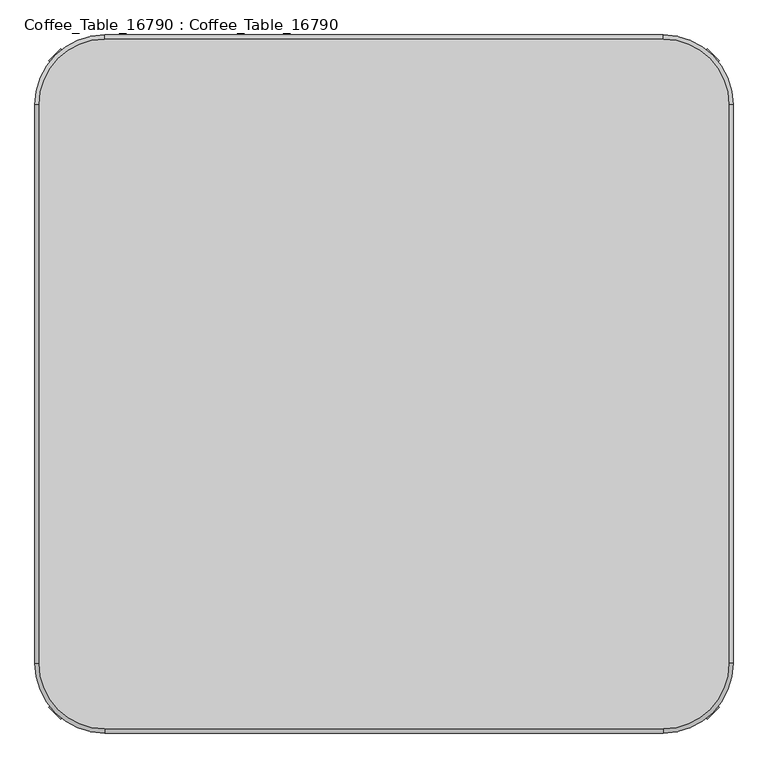
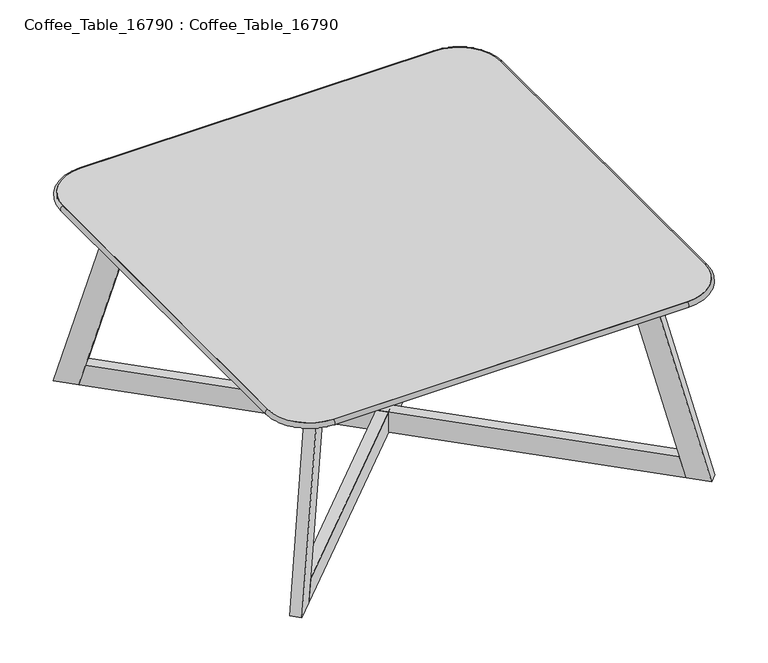
"""IFC4 building model written with IfcOpenShell, lengths in millimetres: furniture geometry, Coffee_Table_16790 : Coffee_Table_16790."""

from ifc_helpers import new_model, si_unit, point, frame, frame_2d, origin, place, context, project, spatial, polyline, circle_curve, ellipse_curve, trimmed, segment, composite_curve, outline, extrude, source, transform, mapped, element, save
from ifc_brep_helpers import plane_surface, cylinder_surface, revolved_surface, advanced_brep


def coffee_table_16790_coffee_table_16790_723536ea(model_context):
    return source(origin(), model_context, "Body", "SolidModel", [
        extrude(outline(composite_curve([segment(trimmed(circle_curve(frame_2d((400.0, 400.0)), 94.0), [point((400.0, 494.0))], [point((494.0, 400.0))], False, "CARTESIAN"), True, "CONTINUOUS"), segment(polyline([(494.0, 400.0), (494.0, -400.0)]), True, "CONTINUOUS"), segment(trimmed(circle_curve(frame_2d((400.0, -400.0)), 94.0), [point((494.0, -400.0))], [point((400.0, -494.0))], False, "CARTESIAN"), True, "CONTINUOUS"), segment(polyline([(400.0, -494.0), (-400.0, -494.0)]), True, "CONTINUOUS"), segment(trimmed(circle_curve(frame_2d((-400.0, -400.0)), 94.0), [point((-400.0, -494.0))], [point((-494.0, -400.0))], False, "CARTESIAN"), True, "CONTINUOUS"), segment(polyline([(-494.0, -400.0), (-494.0, 400.0)]), True, "CONTINUOUS"), segment(trimmed(circle_curve(frame_2d((-400.0, 400.0)), 94.0), [point((-494.0, 400.0))], [point((-400.0, 494.0))], False, "CARTESIAN"), True, "CONTINUOUS"), segment(polyline([(-400.0, 494.0), (400.0, 494.0)]), True, "CONTINUOUS")], self_intersect=False)), frame((0.0, 0.0, 448.0), z_axis=(0.0, 0.0, 1.0), x_axis=(1.0, 0.0, 0.0)), (0.0, 0.0, 1.0), 12.0),
        advanced_brep(
        [(-494.0, 400.0, 460.0), (-494.0, 400.0, 448.0), (-494.0, -400.0, 448.0), (-494.0, -400.0, 460.0), (-400.0, -494.0, 460.0), (-400.0, -494.0, 448.0), (400.0, -494.0, 448.0), (400.0, -494.0, 460.0), (494.0, -400.0, 460.0), (494.0, -400.0, 448.0), (494.0, 400.0, 448.0), (494.0, 400.0, 460.0), (400.0, 494.0, 460.0), (400.0, 494.0, 448.0), (-400.0, 494.0, 448.0), (-400.0, 494.0, 460.0)],
        [
            (0, 1, circle_curve(frame((-494.0, 400.0, 454.0), z_axis=(0.0, -1.0, 0.0), x_axis=(1.0, 0.0, 0.0)), 6.0)),
            (1, 2),
            (2, 3, circle_curve(frame((-494.0, -400.0, 454.0), z_axis=(0.0, 1.0, 0.0), x_axis=(1.0, 0.0, 0.0)), 6.0)),
            (3, 0),
            (1, 0),
            (3, 2),
            (4, 3, circle_curve(frame((-400.0, -400.0, 460.0), z_axis=(0.0, 0.0, -1.0), x_axis=(-1.0, 0.0, 0.0)), 94.0)),
            (2, 5, circle_curve(frame((-400.0, -400.0, 448.0), z_axis=(0.0, 0.0, 1.0), x_axis=(-1.0, 0.0, 0.0)), 94.0)),
            (5, 4, circle_curve(frame((-400.0, -494.0, 454.0), z_axis=(-1.0, 0.0, 0.0), x_axis=(0.0, 1.0, 0.0)), 6.0)),
            (4, 5),
            (5, 6),
            (6, 7, circle_curve(frame((400.0, -494.0, 454.0), z_axis=(-1.0, 0.0, 0.0), x_axis=(0.0, 1.0, 0.0)), 6.0)),
            (7, 4),
            (7, 6),
            (8, 7, circle_curve(frame((400.0, -400.0, 460.0), z_axis=(0.0, 0.0, -1.0), x_axis=(0.0, -1.0, 0.0)), 94.0)),
            (6, 9, circle_curve(frame((400.0, -400.0, 448.0), z_axis=(0.0, 0.0, 1.0), x_axis=(0.0, -1.0, 0.0)), 94.0)),
            (9, 8, circle_curve(frame((494.0, -400.0, 454.0), z_axis=(0.0, -1.0, 0.0), x_axis=(-1.0, 0.0, 0.0)), 6.0)),
            (8, 9),
            (9, 10),
            (10, 11, circle_curve(frame((494.0, 400.0, 454.0), z_axis=(0.0, -1.0, 0.0), x_axis=(-1.0, 0.0, 0.0)), 6.0)),
            (11, 8),
            (11, 10),
            (12, 11, circle_curve(frame((400.0, 400.0, 460.0), z_axis=(0.0, 0.0, -1.0), x_axis=(1.0, 0.0, 0.0)), 94.0)),
            (10, 13, circle_curve(frame((400.0, 400.0, 448.0), z_axis=(0.0, 0.0, 1.0), x_axis=(1.0, 0.0, 0.0)), 94.0)),
            (13, 12, circle_curve(frame((400.0, 494.0, 454.0), z_axis=(1.0, 0.0, 0.0), x_axis=(0.0, -1.0, 0.0)), 6.0)),
            (12, 13),
            (13, 14),
            (14, 15, circle_curve(frame((-400.0, 494.0, 454.0), z_axis=(1.0, 0.0, 0.0), x_axis=(0.0, -1.0, 0.0)), 6.0)),
            (15, 12),
            (15, 14),
            (0, 15, circle_curve(frame((-400.0, 400.0, 460.0), z_axis=(0.0, 0.0, -1.0), x_axis=(0.0, 1.0, 0.0)), 94.0)),
            (14, 1, circle_curve(frame((-400.0, 400.0, 448.0), z_axis=(0.0, 0.0, 1.0), x_axis=(0.0, 1.0, 0.0)), 94.0)),
        ],
        [
            cylinder_surface(frame((-494.0, 400.0, 454.0), z_axis=(0.0, 1.0, 0.0), x_axis=(1.0, 0.0, 0.0)), 6.0),
            plane_surface(frame((-494.0, 400.0, 460.0), z_axis=(1.0, 0.0, 0.0), x_axis=(0.0, -1.0, 0.0))),
            revolved_surface(trimmed(ellipse_curve(frame((-494.0, -400.0, 454.0), z_axis=(0.0, 1.0, 0.0), x_axis=(1.0, 0.0, 0.0)), 6.0, 6.0), [point((-494.0, -400.0, 448.0))], [point((-494.0, -400.0, 460.0))], True, "CARTESIAN"), (-400.0, -400.0, 0.0), (0.0, 0.0, 1.0)),
            revolved_surface(polyline([(-494.0, -400.0, 460.0), (-494.0, -400.0, 448.0)]), (-400.0, -400.0, 0.0), (0.0, 0.0, 1.0)),
            cylinder_surface(frame((-400.0, -494.0, 454.0), z_axis=(-1.0, 0.0, 0.0), x_axis=(0.0, 1.0, 0.0)), 6.0),
            plane_surface(frame((-400.0, -494.0, 460.0), z_axis=(0.0, 1.0, 0.0), x_axis=(1.0, 0.0, 0.0))),
            revolved_surface(trimmed(ellipse_curve(frame((400.0, -494.0, 454.0), z_axis=(-1.0, 0.0, 0.0), x_axis=(0.0, 1.0, 0.0)), 6.0, 6.0), [point((400.0, -494.0, 448.0))], [point((400.0, -494.0, 460.0))], True, "CARTESIAN"), (400.0, -400.0, 0.0), (0.0, 0.0, 1.0)),
            revolved_surface(polyline([(400.0, -494.0, 460.0), (400.0, -494.0, 448.0)]), (400.0, -400.0, 0.0), (0.0, 0.0, 1.0)),
            cylinder_surface(frame((494.0, -400.0, 454.0), z_axis=(0.0, -1.0, 0.0), x_axis=(-1.0, 0.0, 0.0)), 6.0),
            plane_surface(frame((494.0, -400.0, 460.0), z_axis=(-1.0, 0.0, 0.0), x_axis=(0.0, 1.0, 0.0))),
            revolved_surface(trimmed(ellipse_curve(frame((494.0, 400.0, 454.0), z_axis=(0.0, -1.0, 0.0), x_axis=(-1.0, 0.0, 0.0)), 6.0, 6.0), [point((494.0, 400.0, 448.0))], [point((494.0, 400.0, 460.0))], True, "CARTESIAN"), (400.0, 400.0, 0.0), (0.0, 0.0, 1.0)),
            revolved_surface(polyline([(494.0, 400.0, 460.0), (494.0, 400.0, 448.0)]), (400.0, 400.0, 0.0), (0.0, 0.0, 1.0)),
            cylinder_surface(frame((400.0, 494.0, 454.0), z_axis=(1.0, 0.0, 0.0), x_axis=(0.0, -1.0, 0.0)), 6.0),
            plane_surface(frame((400.0, 494.0, 460.0), z_axis=(0.0, -1.0, 0.0), x_axis=(-1.0, 0.0, 0.0))),
            revolved_surface(trimmed(ellipse_curve(frame((-400.0, 494.0, 454.0), z_axis=(1.0, 0.0, 0.0), x_axis=(0.0, -1.0, 0.0)), 6.0, 6.0), [point((-400.0, 494.0, 448.0))], [point((-400.0, 494.0, 460.0))], True, "CARTESIAN"), (-400.0, 400.0, 0.0), (0.0, 0.0, 1.0)),
            revolved_surface(polyline([(-400.0, 494.0, 460.0), (-400.0, 494.0, 448.0)]), (-400.0, 400.0, 0.0), (0.0, 0.0, 1.0)),
        ],
        [
            (0, [[1, 2, 3, 4]]),
            (1, [[5, -4, 6, -2]]),
            (2, [[7, -3, 8, 9]]),
            (3, [[-8, -6, -7, 10]]),
            (4, [[-9, 11, 12, 13]]),
            (5, [[-10, -13, 14, -11]]),
            (6, [[15, -12, 16, 17]]),
            (7, [[-16, -14, -15, 18]]),
            (8, [[-17, 19, 20, 21]]),
            (9, [[-18, -21, 22, -19]]),
            (10, [[23, -20, 24, 25]]),
            (11, [[-24, -22, -23, 26]]),
            (12, [[-25, 27, 28, 29]]),
            (13, [[-26, -29, 30, -27]]),
            (14, [[31, -28, 32, -1]]),
            (15, [[-32, -30, -31, -5]]),
        ],
    ),
        extrude(outline(polyline([(465.1118145, 0.0), (451.1609217, -50.0), (-8.7599128, -50.0), (5.1909801, 0.0), (465.1118145, 0.0)])), frame((-392.0907102, 374.4130406, 448.0), z_axis=(0.7071067811865499, 0.7071067811865451, 0.0), x_axis=(-0.19003677156810073, 0.19003677156810195, -0.9632092456491199)), (0.0, 0.0, 1.0), 25.0),
        extrude(outline(polyline([(106.5958732, -1284.9211337), (-286.886684, -1046.8063481), (-272.9357912, -996.8063481), (120.546766, -1234.9211337), (106.5958732, -1284.9211337)])), frame((-392.0907102, 374.4130406, 448.0), z_axis=(0.7071067811865499, 0.7071067811865451, 0.0), x_axis=(-0.19003677156810073, 0.19003677156810195, -0.9632092456491199)), (0.0, 0.0, 1.0), 25.0),
        extrude(outline(polyline([(1230.1803986, 0.0), (1216.7427695, -48.1604623), (13.437629, -48.1604623), (0.0, 0.0), (1230.1803986, 0.0)])), frame((-443.7732857, 426.0956162, 0.0), z_axis=(0.7071067811865499, 0.7071067811865451, 0.0), x_axis=(0.7071067811865451, -0.7071067811865499, 0.0)), (0.0, 0.0, 1.0), 25.0),
        extrude(outline(polyline([(0.0, 0.0), (-123.6049107, -443.0), (-175.5147114, -443.0), (-51.9098007, 0.0), (0.0, 0.0)])), frame((480.4790578, 462.8013883, 0.0), z_axis=(-0.7071067811865499, 0.7071067811865451, 0.0), x_axis=(0.7071067811865451, 0.7071067811865499, 0.0)), (0.0, 0.0, 1.0), 25.0),
        extrude(outline(polyline([(-1334.0, 0.0), (-1282.0901993, 0.0), (-1158.4852886, -443.0), (-1210.3950893, -443.0), (-1334.0, 0.0)])), frame((480.4790578, 462.8013883, 0.0), z_axis=(-0.7071067811865499, 0.7071067811865451, 0.0), x_axis=(0.7071067811865451, 0.7071067811865499, 0.0)), (0.0, 0.0, 1.0), 25.0),
        extrude(outline(polyline([(0.0, 0.0), (-330.6141556, -1184.9211337), (-373.3913607, -1159.0346367), (-50.0, 0.0), (0.0, 0.0)])), frame((-426.0956162, -443.7732857, 0.0), z_axis=(-0.7071067811865499, 0.7071067811865452, 0.0), x_axis=(-0.19003677156810203, -0.1900367715681033, -0.9632092456491194)), (0.0, 0.0, 1.0), 25.0),
        extrude(outline(composite_curve([segment(trimmed(circle_curve(frame_2d((-365.8854664, 365.8854664)), 10.0), [point((-375.8854664, 365.8854664))], [point((-355.8854664, 365.8854664))], False, "CARTESIAN"), True, "CONTINUOUS"), segment(trimmed(circle_curve(frame_2d((-365.8854664, 365.8854664)), 10.0), [point((-355.8854664, 365.8854664))], [point((-375.8854664, 365.8854664))], False, "CARTESIAN"), True, "CONTINUOUS")], self_intersect=False)), frame((0.0, 0.0, 443.0), z_axis=(0.0, 0.0, 1.0), x_axis=(1.0, 0.0, 0.0)), (0.0, 0.0, 1.0), 5.0),
        extrude(outline(composite_curve([segment(trimmed(circle_curve(frame_2d((365.8854664, 365.8854664)), 10.0), [point((375.8854664, 365.8854664))], [point((355.8854664, 365.8854664))], False, "CARTESIAN"), True, "CONTINUOUS"), segment(trimmed(circle_curve(frame_2d((365.8854664, 365.8854664)), 10.0), [point((355.8854664, 365.8854664))], [point((375.8854664, 365.8854664))], False, "CARTESIAN"), True, "CONTINUOUS")], self_intersect=False)), frame((0.0, 0.0, 443.0), z_axis=(0.0, 0.0, 1.0), x_axis=(1.0, 0.0, 0.0)), (0.0, 0.0, 1.0), 5.0),
        extrude(outline(composite_curve([segment(trimmed(circle_curve(frame_2d((-365.8854664, -365.8854664)), 10.0), [point((-375.8854664, -365.8854664))], [point((-355.8854664, -365.8854664))], False, "CARTESIAN"), True, "CONTINUOUS"), segment(trimmed(circle_curve(frame_2d((-365.8854664, -365.8854664)), 10.0), [point((-355.8854664, -365.8854664))], [point((-375.8854664, -365.8854664))], False, "CARTESIAN"), True, "CONTINUOUS")], self_intersect=False)), frame((0.0, 0.0, 443.0), z_axis=(0.0, 0.0, 1.0), x_axis=(1.0, 0.0, 0.0)), (0.0, 0.0, 1.0), 5.0),
        extrude(outline(composite_curve([segment(trimmed(circle_curve(frame_2d((365.8854664, -365.8854664)), 10.0), [point((375.8854664, -365.8854664))], [point((355.8854664, -365.8854664))], False, "CARTESIAN"), True, "CONTINUOUS"), segment(trimmed(circle_curve(frame_2d((365.8854664, -365.8854664)), 10.0), [point((355.8854664, -365.8854664))], [point((375.8854664, -365.8854664))], False, "CARTESIAN"), True, "CONTINUOUS")], self_intersect=False)), frame((0.0, 0.0, 443.0), z_axis=(0.0, 0.0, 1.0), x_axis=(1.0, 0.0, 0.0)), (0.0, 0.0, 1.0), 5.0),
    ])


if __name__ == "__main__":
    model = new_model("IFC4")
    model_context = context("Model", 3, world=origin())
    ifc_project = project(units=[si_unit("LENGTHUNIT", "METRE", prefix="MILLI")], contexts=[model_context])
    site = spatial("IfcSite", under=ifc_project)
    building = spatial("IfcBuilding", under=site)
    placement = place(None, origin())
    coffee_table_16790_coffee_table_16790_shape = coffee_table_16790_coffee_table_16790_723536ea(model_context)
    element("IfcFurniture", 1, ObjectType="Coffee_Table_16790 : Coffee_Table_16790", at=placement, inside=building, context=model_context, shape_type="MappedRepresentation", body=[
        mapped(coffee_table_16790_coffee_table_16790_shape, transform((0.0, 0.0, 0.0), x_axis=(1.0, 0.0, 0.0), y_axis=(0.0, 1.0, 0.0), z_axis=(0.0, 0.0, 1.0))),
    ])
    save(model, "model.ifc")

# Revit data of these elements
# Type "Coffee_Table_16790 : Coffee_Table_16790"
#   Coffee Table - Stand = Coffee Table - Stand
#   Coffee Table - Glass = Coffee Table - Glass
#   Default Elevation = 0
# Element 1 (IfcFurniture, "Coffee_Table_16790 : Coffee_Table_16790")
#   Materials on its faces: "Coffee Table - Stand", "Coffee Table - Glass"
# Materials
#   "Coffee Table - Stand": class "Generic", colour RGB 120 120 120, transparency 0, Cost = 0
#   "Coffee Table - Glass": class "Generic", colour RGB 120 120 120, transparency 0, Cost = 0
